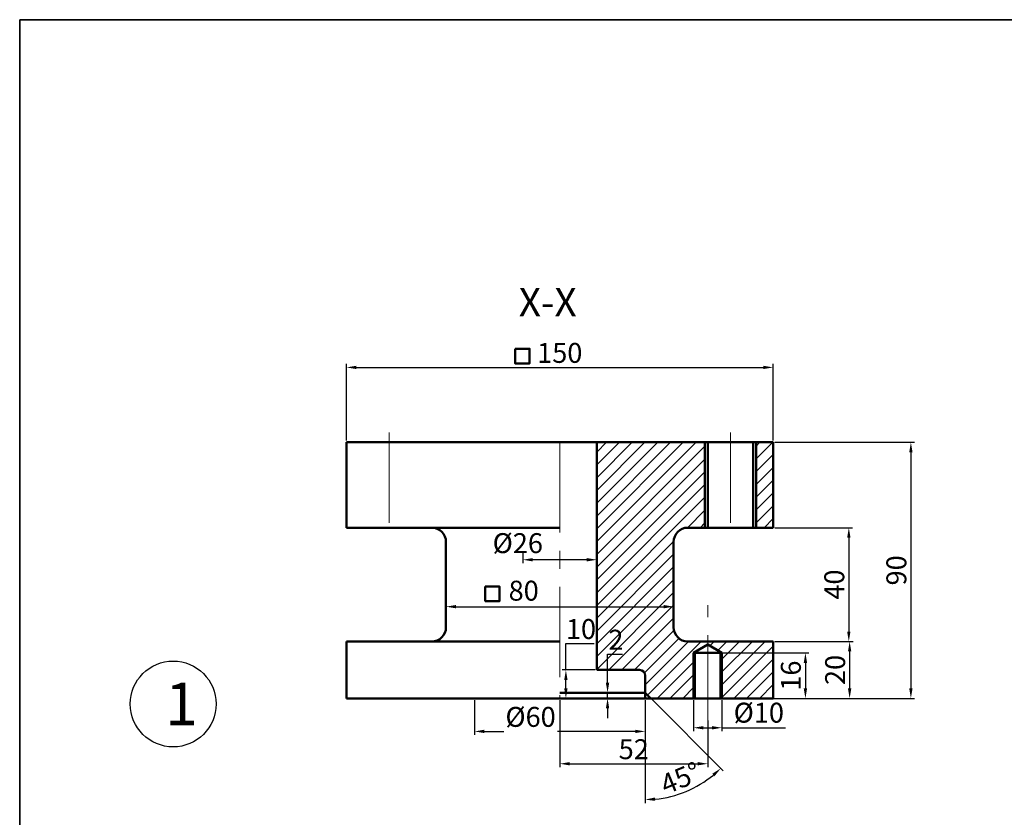
# Model space of a CAD drawing. Units: millimetres. Extents: x -5 to 1372, y -339 to 395.
# Tile 2 of 6: x -5 to 341, y 114 to 395. Entities that reach past the tile are written whole.
import ezdxf

# ---------------------------------------------------------------- set-up
doc = ezdxf.new("R2010")
doc.units = ezdxf.units.MM
doc.linetypes.add('CENTER', pattern=[50.8, 31.75, -6.35, 6.35, -6.35])
for name, color, linetype, lineweight in [('M-CNTR', 1, 'CENTER', 18), ('M-DIMS', 2, 'Continuous', 25), ('M-HATC', 8, 'Continuous', 18), ('M-OUTL', 7, 'Continuous', 50), ('M-TEXT', 3, 'Continuous', 25), ('M-TTLB', 7, 'Continuous', 35)]:
    doc.layers.add(name, color=color, linetype=linetype, lineweight=lineweight)
doc.styles.get("Standard").update_dxf_attribs({"font": 'arial.ttf'})
doc.dimstyles.new('ISO-25', dxfattribs={"dimtxt": 7, "dimasz": 3.5, "dimexe": 1.25, "dimexo": 0.625, "dimtad": 1, "dimtoh": 1, "dimtxsty": 'Standard', "dimcen": 2.5, "dimadec": 0, "dimazin": 0, "dimtfac": 1, "dimtmove": 0, "dimatfit": 3, "dimfxl": 1, "dimarcsym": 0})

# ---------------------------------------------------------------- blocks, each defined once
blk = doc.blocks.new('*U1')
at = {"layer": 'M-CNTR', "color": 0, "transparency": 16777216}
blk.add_line((0, 18.5), (0, -18.5), dxfattribs=at)
blk = doc.blocks.new('*U2')
at = {"layer": 'M-CNTR', "color": 0, "transparency": 16777216}
blk.add_line((0, -17.55), (0, 24.76), dxfattribs=at)
blk = doc.blocks.new('*U3')
at = {"layer": 'M-CNTR', "color": 0, "transparency": 16777216}
blk.add_line((0, 18.5), (0, -18.5), dxfattribs=at)
blk = doc.blocks.new('*D4')
at = {"layer": 'Defpoints', "color": 0, "transparency": 16777216}
for p in [(259.85, 272.53), (109.85, 246.21), (259.85, 246.21)]:
    blk.add_point(p, dxfattribs=at)
at = {"layer": 'M-DIMS', "color": 0, "lineweight": -2, "transparency": 16777216}
for p, q in [((109.85, 246.84), (109.85, 273.78)), ((259.85, 246.84), (259.85, 273.78)), ((113.35, 272.53), (256.35, 272.53))]:
    blk.add_line(p, q, dxfattribs=at)
at = {"layer": 'M-DIMS', "color": 0, "transparency": 16777216}
for points in [[(113.35, 273.11), (113.35, 271.95), (109.85, 272.53)], [(256.35, 273.11), (256.35, 271.95), (259.85, 272.53)]]:
    blk.add_solid(points, dxfattribs=at)
at = {"layer": 'M-DIMS', "color": 0, "transparency": 16777216, "insert": (184.85, 276.73), "char_height": 7, "attachment_point": 5}
blk.add_mtext('150', dxfattribs=at)
blk = doc.blocks.new('*D5')
at = {"layer": 'Defpoints', "color": 0, "transparency": 16777216}
for p in [(144.85, 191.43), (224.85, 191.43), (224.85, 188.45)]:
    blk.add_point(p, dxfattribs=at)
at = {"layer": 'M-DIMS', "color": 0, "lineweight": -2, "transparency": 16777216}
for p, q in [((144.85, 190.8), (144.85, 187.2)), ((224.85, 190.8), (224.85, 187.2)), ((148.35, 188.45), (221.35, 188.45))]:
    blk.add_line(p, q, dxfattribs=at)
at = {"layer": 'M-DIMS', "color": 0, "transparency": 16777216}
for points in [[(148.35, 189.03), (148.35, 187.87), (144.85, 188.45)], [(221.35, 189.03), (221.35, 187.87), (224.85, 188.45)]]:
    blk.add_solid(points, dxfattribs=at)
at = {"layer": 'M-DIMS', "color": 0, "transparency": 16777216, "insert": (172.17, 193.16), "char_height": 7, "attachment_point": 5}
blk.add_mtext('80', dxfattribs=at)
blk = doc.blocks.new('*D6')
at = {"layer": 'Defpoints', "color": 0, "transparency": 16777216}
for p in [(171.85, 208.35), (197.85, 208.35), (171.85, 204.94)]:
    blk.add_point(p, dxfattribs=at)
at = {"layer": 'M-DIMS', "color": 0, "lineweight": -2, "transparency": 16777216}
for p, q in [((171.85, 207.73), (171.85, 203.69)), ((197.85, 207.73), (197.85, 203.69)), ((194.35, 204.94), (175.35, 204.94))]:
    blk.add_line(p, q, dxfattribs=at)
at = {"layer": 'M-DIMS', "color": 0, "transparency": 16777216}
for points in [[(175.35, 205.52), (175.35, 204.36), (171.85, 204.94)], [(194.35, 205.52), (194.35, 204.36), (197.85, 204.94)]]:
    blk.add_solid(points, dxfattribs=at)
at = {"layer": 'M-DIMS', "color": 0, "transparency": 16777216, "insert": (170.1, 209.87), "char_height": 7, "attachment_point": 5}
blk.add_mtext('%%C26', dxfattribs=at)
blk = doc.blocks.new('*D7')
at = {"layer": 'Defpoints', "color": 0, "transparency": 16777216}
for p in [(259.85, 246.21), (259.85, 156.21), (308.24, 156.21)]:
    blk.add_point(p, dxfattribs=at)
at = {"layer": 'M-DIMS', "color": 0, "lineweight": -2, "transparency": 16777216}
for p, q in [((260.48, 246.21), (309.49, 246.21)), ((308.24, 242.71), (308.24, 159.71)), ((260.48, 156.21), (309.49, 156.21))]:
    blk.add_line(p, q, dxfattribs=at)
at = {"layer": 'M-DIMS', "color": 0, "transparency": 16777216}
for points in [[(307.66, 242.71), (308.82, 242.71), (308.24, 246.21)], [(307.66, 159.71), (308.82, 159.71), (308.24, 156.21)]]:
    blk.add_solid(points, dxfattribs=at)
at = {"layer": 'M-DIMS', "color": 0, "transparency": 16777216, "insert": (304.04, 201.21), "char_height": 7, "attachment_point": 5, "rotation": 90}
blk.add_mtext('90', dxfattribs=at)
blk = doc.blocks.new('*D8')
at = {"layer": 'Defpoints', "color": 0, "transparency": 16777216}
for p in [(259.85, 176.21), (259.85, 156.21), (286.72, 156.21)]:
    blk.add_point(p, dxfattribs=at)
at = {"layer": 'M-DIMS', "color": 0, "lineweight": -2, "transparency": 16777216}
for p, q in [((260.48, 176.21), (287.97, 176.21)), ((286.72, 172.71), (286.72, 159.71)), ((260.48, 156.21), (287.97, 156.21))]:
    blk.add_line(p, q, dxfattribs=at)
at = {"layer": 'M-DIMS', "color": 0, "transparency": 16777216}
for points in [[(286.13, 172.71), (287.3, 172.71), (286.72, 176.21)], [(286.13, 159.71), (287.3, 159.71), (286.72, 156.21)]]:
    blk.add_solid(points, dxfattribs=at)
at = {"layer": 'M-DIMS', "color": 0, "transparency": 16777216, "insert": (282.52, 166.21), "char_height": 7, "attachment_point": 5, "rotation": 90}
blk.add_mtext('20', dxfattribs=at)
blk = doc.blocks.new('*D9')
at = {"layer": 'Defpoints', "color": 0, "transparency": 16777216}
for p in [(241.35, 172.21), (241.35, 156.21), (271.17, 156.21)]:
    blk.add_point(p, dxfattribs=at)
at = {"layer": 'M-DIMS', "color": 0, "lineweight": -2, "transparency": 16777216}
for p, q in [((241.98, 172.21), (272.42, 172.21)), ((271.17, 168.71), (271.17, 159.71)), ((241.98, 156.21), (272.42, 156.21))]:
    blk.add_line(p, q, dxfattribs=at)
at = {"layer": 'M-DIMS', "color": 0, "transparency": 16777216}
for points in [[(270.59, 168.71), (271.76, 168.71), (271.17, 172.21)], [(270.59, 159.71), (271.76, 159.71), (271.17, 156.21)]]:
    blk.add_solid(points, dxfattribs=at)
at = {"layer": 'M-DIMS', "color": 0, "transparency": 16777216, "insert": (266.97, 164.21), "char_height": 7, "attachment_point": 5, "rotation": 90}
blk.add_mtext('16', dxfattribs=at)
blk = doc.blocks.new('*D10')
at = {"layer": 'Defpoints', "color": 0, "transparency": 16777216}
for p in [(259.85, 216.21), (274.22, 176.21), (286.43, 176.21)]:
    blk.add_point(p, dxfattribs=at)
at = {"layer": 'M-DIMS', "color": 0, "lineweight": -2, "transparency": 16777216}
for p, q in [((260.48, 216.21), (287.68, 216.21)), ((286.43, 212.71), (286.43, 179.71)), ((274.85, 176.21), (287.68, 176.21))]:
    blk.add_line(p, q, dxfattribs=at)
at = {"layer": 'M-DIMS', "color": 0, "transparency": 16777216}
for points in [[(285.84, 212.71), (287.01, 212.71), (286.43, 216.21)], [(285.84, 179.71), (287.01, 179.71), (286.43, 176.21)]]:
    blk.add_solid(points, dxfattribs=at)
at = {"layer": 'M-DIMS', "color": 0, "transparency": 16777216, "insert": (282.23, 196.21), "char_height": 7, "attachment_point": 5, "rotation": 90}
blk.add_mtext('40', dxfattribs=at)
blk = doc.blocks.new('*D11')
at = {"layer": 'Defpoints', "color": 0, "transparency": 16777216}
for p in [(231.85, 156.21), (241.85, 156.21), (241.85, 145.9)]:
    blk.add_point(p, dxfattribs=at)
at = {"layer": 'M-DIMS', "color": 0, "lineweight": -2, "transparency": 16777216}
for p, q in [((231.85, 155.59), (231.85, 144.65)), ((241.85, 155.59), (241.85, 144.65)), ((235.35, 145.9), (238.35, 145.9)), ((241.85, 145.9), (264.22, 145.9))]:
    blk.add_line(p, q, dxfattribs=at)
at = {"layer": 'M-DIMS', "color": 0, "transparency": 16777216}
for points in [[(235.35, 146.48), (235.35, 145.31), (231.85, 145.9)], [(238.35, 146.48), (238.35, 145.31), (241.85, 145.9)]]:
    blk.add_solid(points, dxfattribs=at)
at = {"layer": 'M-DIMS', "color": 0, "transparency": 16777216, "insert": (254.79, 150.29), "char_height": 7, "attachment_point": 5}
blk.add_mtext('%%C10', dxfattribs=at)
blk = doc.blocks.new('*D12')
at = {"layer": 'Defpoints', "color": 0, "transparency": 16777216}
for p in [(197.85, 166.21), (187, 156.21), (197.85, 156.21)]:
    blk.add_point(p, dxfattribs=at)
at = {"layer": 'M-DIMS', "color": 0, "lineweight": -2, "transparency": 16777216}
for p, q in [((187, 166.21), (187, 175.5)), ((187, 175.5), (196.97, 175.5)), ((197.23, 166.21), (185.75, 166.21)), ((187, 159.71), (187, 162.71)), ((197.23, 156.21), (185.75, 156.21))]:
    blk.add_line(p, q, dxfattribs=at)
at = {"layer": 'M-DIMS', "color": 0, "transparency": 16777216}
for points in [[(186.42, 162.71), (187.58, 162.71), (187, 166.21)], [(186.42, 159.71), (187.58, 159.71), (187, 156.21)]]:
    blk.add_solid(points, dxfattribs=at)
at = {"layer": 'M-DIMS', "color": 0, "transparency": 16777216, "insert": (192.3, 179.69), "char_height": 7, "attachment_point": 5}
blk.add_mtext('10', dxfattribs=at)
blk = doc.blocks.new('*D13')
at = {"layer": 'Defpoints', "color": 0, "transparency": 16777216}
for p in [(184.85, 156.21), (236.85, 149.07), (236.85, 133.25)]:
    blk.add_point(p, dxfattribs=at)
at = {"layer": 'M-DIMS', "color": 0, "lineweight": -2, "transparency": 16777216}
for p, q in [((184.85, 155.59), (184.85, 132)), ((236.85, 148.44), (236.85, 132)), ((188.35, 133.25), (233.35, 133.25))]:
    blk.add_line(p, q, dxfattribs=at)
at = {"layer": 'M-DIMS', "color": 0, "transparency": 16777216}
for points in [[(188.35, 133.83), (188.35, 132.67), (184.85, 133.25)], [(233.35, 133.83), (233.35, 132.67), (236.85, 133.25)]]:
    blk.add_solid(points, dxfattribs=at)
at = {"layer": 'M-DIMS', "color": 0, "transparency": 16777216, "insert": (210.85, 137.45), "char_height": 7, "attachment_point": 5}
blk.add_mtext('52', dxfattribs=at)
blk = doc.blocks.new('*D14')
at = {"layer": 'Defpoints', "color": 0, "transparency": 16777216}
for p in [(154.85, 156.21), (214.85, 156.21), (154.85, 144.61)]:
    blk.add_point(p, dxfattribs=at)
at = {"layer": 'M-DIMS', "color": 0, "lineweight": -2, "transparency": 16777216}
for p, q in [((154.85, 155.59), (154.85, 143.36)), ((214.85, 155.59), (214.85, 143.36)), ((158.35, 144.61), (165.15, 144.61)), ((211.35, 144.61), (184.02, 144.61))]:
    blk.add_line(p, q, dxfattribs=at)
at = {"layer": 'M-DIMS', "color": 0, "transparency": 16777216}
for points in [[(158.35, 145.2), (158.35, 144.03), (154.85, 144.61)], [(211.35, 145.2), (211.35, 144.03), (214.85, 144.61)]]:
    blk.add_solid(points, dxfattribs=at)
at = {"layer": 'M-DIMS', "color": 0, "transparency": 16777216, "insert": (174.59, 148.81), "char_height": 7, "attachment_point": 5}
blk.add_mtext('%%C60', dxfattribs=at)
blk = doc.blocks.new('*D15')
at = {"layer": 'Defpoints', "color": 0, "transparency": 16777216}
for p in [(201.64, 158.21), (202.25, 158.21), (202.25, 156.21)]:
    blk.add_point(p, dxfattribs=at)
at = {"layer": 'M-DIMS', "color": 0, "lineweight": -2, "transparency": 16777216}
for p, q in [((201.64, 161.71), (201.64, 171.79)), ((201.64, 171.79), (206.9, 171.79)), ((201.63, 158.21), (200.39, 158.21)), ((201.63, 156.21), (200.39, 156.21)), ((201.64, 156.21), (201.64, 158.21)), ((201.64, 152.71), (201.64, 149.21))]:
    blk.add_line(p, q, dxfattribs=at)
at = {"layer": 'M-DIMS', "color": 0, "transparency": 16777216}
for points in [[(201.05, 161.71), (202.22, 161.71), (201.64, 158.21)], [(201.05, 152.71), (202.22, 152.71), (201.64, 156.21)]]:
    blk.add_solid(points, dxfattribs=at)
at = {"layer": 'M-DIMS', "color": 0, "transparency": 16777216, "insert": (204.58, 175.93), "char_height": 7, "attachment_point": 5}
blk.add_mtext('2', dxfattribs=at)
blk = doc.blocks.new('*D16')
at = {"layer": 'Defpoints', "color": 0, "transparency": 16777216}
for p in [(214.85, 164.21), (214.85, 158.21), (214.85, 156.21), (216.85, 156.21), (224.58, 121.92)]:
    blk.add_point(p, dxfattribs=at)
at = {"layer": 'M-DIMS', "color": 0, "lineweight": -2, "transparency": 16777216}
for p, q in [((217.3, 155.77), (242.31, 130.76)), ((214.85, 155.59), (214.85, 119.39))]:
    blk.add_line(p, q, dxfattribs=at)
blk.add_arc((214.85, 158.21), 37.57, 275.3393, 309.6607, dxfattribs=at)
at = {"layer": 'M-DIMS', "color": 0, "transparency": 16777216}
for points in [[(238.44, 129.72), (239.23, 128.86), (241.42, 131.64)], [(218.38, 120.22), (218.32, 121.39), (214.85, 120.64)]]:
    blk.add_solid(points, dxfattribs=at)
at = {"layer": 'M-DIMS', "color": 0, "transparency": 16777216, "insert": (227.63, 127.37), "char_height": 7, "attachment_point": 5, "rotation": 22.5}
blk.add_mtext('45°', dxfattribs=at)

msp = doc.modelspace()

# ---------------------------------------------------------------- hatches: boundary and pattern name
at = {"layer": 'M-HATC'}
h = msp.add_hatch(dxfattribs=at)
h.set_pattern_fill('ANSI31', color=256)
h.paths.add_polyline_path([(235.854, 246.212), (197.854, 246.212), (197.854, 166.212), (212.854, 166.212, -0.4142136), (214.854, 164.212), (214.854, 158.212), (216.854, 156.212), (231.854, 156.212), (231.854, 172.212), (236.854, 175.099), (236.854, 176.212), (229.854, 176.212, -0.4142136), (224.854, 181.212), (224.854, 211.212, -0.4142136), (229.854, 216.212), (235.854, 216.212)])
h.paths.add_polyline_path([(259.854, 246.212), (253.854, 246.212), (253.854, 216.212), (259.854, 216.212)])
h.paths.add_polyline_path([(259.854, 176.212), (236.854, 176.212), (236.854, 175.099), (241.854, 172.212), (241.854, 156.212), (259.854, 156.212)])

# ---------------------------------------------------------------- linework, layer by layer
at = {"layer": 'M-CNTR'}
msp.add_line((184.854, 246.212), (184.854, 156.212), dxfattribs=at)
at = {"layer": 'M-OUTL'}
for p, q in [((259.854, 246.212), (109.854, 246.212)), ((109.854, 246.212), (109.854, 216.212)), ((197.854, 246.212), (197.854, 166.212)), ((235.854, 246.212), (235.854, 216.212)), ((236.854, 246.212), (236.854, 216.212)), ((252.854, 246.212), (252.854, 216.212)), ((253.854, 246.212), (253.854, 216.212)), ((259.854, 216.212), (259.854, 246.212)), ((109.854, 216.212), (184.854, 216.212)), ((229.854, 216.212), (259.854, 216.212)), ((144.854, 211.212), (144.854, 181.212)), ((224.854, 211.212), (224.854, 181.212)), ((109.854, 176.212), (109.854, 156.212)), ((184.854, 176.212), (109.854, 176.212)), ((259.854, 176.212), (229.854, 176.212)), ((231.854, 172.212), (236.854, 175.099)), ((241.854, 172.212), (236.854, 175.099)), ((259.854, 156.212), (259.854, 176.212)), ((231.854, 156.212), (231.854, 172.212)), ((231.854, 172.212), (241.854, 172.212)), ((232.354, 156.212), (232.354, 172.212)), ((241.354, 156.212), (241.354, 172.212)), ((241.854, 156.212), (241.854, 172.212)), ((212.854, 166.212), (197.854, 166.212)), ((214.854, 156.212), (214.854, 164.212)), ((109.854, 156.212), (259.854, 156.212)), ((184.854, 158.212), (214.854, 158.212)), ((214.854, 158.212), (216.854, 156.212))]:
    msp.add_line(p, q, dxfattribs=at)
for points in [[(169.159, 279.061), (174.245, 279.061), (174.245, 273.92), (169.159, 273.92)], [(158.641, 195.527), (163.728, 195.527), (163.728, 190.386), (158.641, 190.386)]]:
    msp.add_lwpolyline(points, close=True, dxfattribs=at)
for centre, radius, start, end in [((139.854, 211.212), 5, 0, 90), ((229.854, 211.212), 5, 90, 180), ((139.854, 181.212), 5, 270, 0), ((229.854, 181.212), 5, 180, 270), ((212.854, 164.212), 2, 360, 90)]:
    msp.add_arc(centre, radius, start, end, dxfattribs=at)
at = {"layer": 'M-TEXT'}
msp.add_circle((48.993, 154.249), 15.085, dxfattribs=at)
at = {"layer": 'M-TTLB'}
msp.add_lwpolyline([(-4.944, 394.729), (1371.917, 394.729), (1371.917, -339.365), (-4.944, -339.365)], close=True, dxfattribs=at)

# ---------------------------------------------------------------- block references
at = {"layer": 'M-CNTR'}
for name, p in [('*U3', (124.854, 231.212)), ('*U1', (244.854, 231.212)), ('*U2', (236.854, 164.212))]:
    msp.add_blockref(name, p, dxfattribs=at)

# ---------------------------------------------------------------- texts
at = {"layer": 'M-TEXT', "attachment_point": 1}
for s, width, insert, char_height in [('X-X', 36.96755, (170.43, 300.453), 10), ('1', 32.93052, (46.23, 161.78), 15)]:
    msp.add_mtext_dynamic_manual_height_columns(s, width=width, gutter_width=12.5, heights=[0], dxfattribs=dict(at, insert=insert, char_height=char_height))

# ---------------------------------------------------------------- dimensions: what is measured, and where the dimension line sits
at = {"layer": 'M-DIMS'}
for base, p1, p2, picture, middle in [((259.854, 272.529), (109.854, 246.212), (259.854, 246.212), '*D4', (184.854, 276.728)), ((236.854, 133.249), (184.854, 156.212), (236.854, 149.065), '*D13', (210.854, 137.448))]:
    dim = msp.add_linear_dim(base=base, p1=p1, p2=p2, dimstyle='ISO-25', override={"dimclrd": 0, "dimclre": 0, "dimclrt": 0}, dxfattribs=at)
    dim.commit()
    dim.dimension.update_dxf_attribs({"geometry": picture, "text_midpoint": middle})
for base, p1, p2, picture, middle in [((308.239, 156.212), (259.854, 246.212), (259.854, 156.212), '*D7', (304.04, 201.212)), ((286.426, 176.212), (259.854, 216.212), (274.223, 176.212), '*D10', (282.227, 196.212)), ((286.718, 156.212), (259.854, 176.212), (259.854, 156.212), '*D8', (282.519, 166.212))]:
    dim = msp.add_linear_dim(base=base, p1=p1, p2=p2, angle=90, dimstyle='ISO-25', override={"dimclrd": 0, "dimclre": 0, "dimclrt": 0}, dxfattribs=at)
    dim.commit()
    dim.dimension.update_dxf_attribs({"geometry": picture, "text_midpoint": middle})
for base, p1, p2, picture, middle in [((171.854, 204.941), (197.854, 208.352), (171.854, 208.352), '*D6', (170.103, 209.874)), ((154.854, 144.612), (214.854, 156.212), (154.854, 156.212), '*D14', (174.587, 148.811))]:
    dim = msp.add_linear_dim(base=base, p1=p1, p2=p2, text='%%C<>', dimstyle='ISO-25', override={"dimclrd": 0, "dimclre": 0, "dimclrt": 0, "dimtmove": 2}, dxfattribs=at)
    dim.commit()
    dim.dimension.update_dxf_attribs({"geometry": picture, "text_midpoint": middle, "dimtype": 160})
dim = msp.add_linear_dim(base=(224.854, 188.451), p1=(144.854, 191.428), p2=(224.854, 191.428), dimstyle='ISO-25', override={"dimclrd": 0, "dimclre": 0, "dimclrt": 0, "dimtmove": 2}, dxfattribs=at)
dim.commit()
dim.dimension.update_dxf_attribs({"geometry": '*D5', "text_midpoint": (172.172, 193.161), "dimtype": 160})
for base, p1, p2, picture, middle in [((186.999, 156.212), (197.854, 166.212), (197.854, 156.212), '*D12', (192.296, 175.496)), ((201.637, 158.212), (202.253, 156.212), (202.253, 158.212), '*D15', (204.58, 171.792)), ((271.172, 156.212), (241.354, 172.212), (241.354, 156.212), '*D9', (271.172, 164.212))]:
    dim = msp.add_linear_dim(base=base, p1=p1, p2=p2, angle=90, dimstyle='ISO-25', override={"dimclrd": 0, "dimclre": 0, "dimclrt": 0}, dxfattribs=at)
    dim.commit()
    dim.dimension.update_dxf_attribs({"geometry": picture, "text_midpoint": middle, "dimtype": 160})
dim = msp.add_angular_dim_2l(base=(224.578, 121.92), line1=((214.854, 158.212), (216.854, 156.212)), line2=((214.854, 156.212), (214.854, 164.212)), dimstyle='ISO-25', override={"dimclrd": 0, "dimclre": 0, "dimclrt": 0}, dxfattribs=at)
dim.commit()
dim.dimension.update_dxf_attribs({"geometry": '*D16', "text_midpoint": (227.63, 127.366)})
dim = msp.add_linear_dim(base=(241.854, 145.897), p1=(231.854, 156.212), p2=(241.854, 156.212), text='%%C<>', dimstyle='ISO-25', override={"dimclrd": 0, "dimclre": 0, "dimclrt": 0}, dxfattribs=at)
dim.commit()
dim.dimension.update_dxf_attribs({"geometry": '*D11', "text_midpoint": (254.788, 150.292)})

doc.saveas('drawing.dxf')
